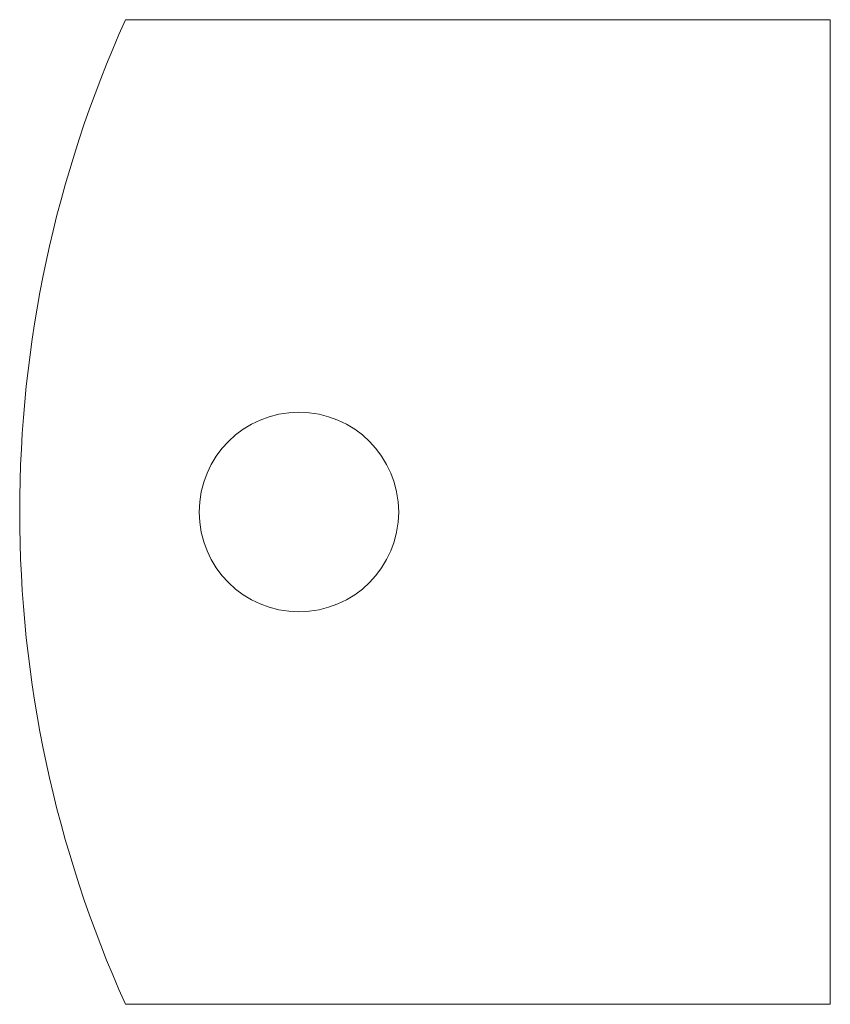
# Model space of a CAD drawing. Units: millimetres. Extents: x 549 to 905, y -110 to 0.
# Tile 2 of 2: x 844 to 905, y -110 to -36. Entities that reach past the tile are written whole.
import ezdxf

# ---------------------------------------------------------------- set-up
doc = ezdxf.new("R2010")
doc.units = ezdxf.units.MM
doc.layers.add('M-CONS', color=8, linetype='Continuous', lineweight=13)

msp = doc.modelspace()

# ---------------------------------------------------------------- linework, layer by layer
at = {"layer": 'M-CONS'}
for p, q in [((904.904, -36.48), (851.904, -36.48)), ((904.904, -36.48), (904.904, -110.48)), ((904.904, -110.48), (851.904, -110.48))]:
    msp.add_line(p, q, dxfattribs=at)
msp.add_circle((864.947, -73.48), 7.5, dxfattribs=at)
msp.add_arc((933.947, -73.48), 90, 155.72535, 204.27465, dxfattribs=at)

doc.saveas('drawing.dxf')
